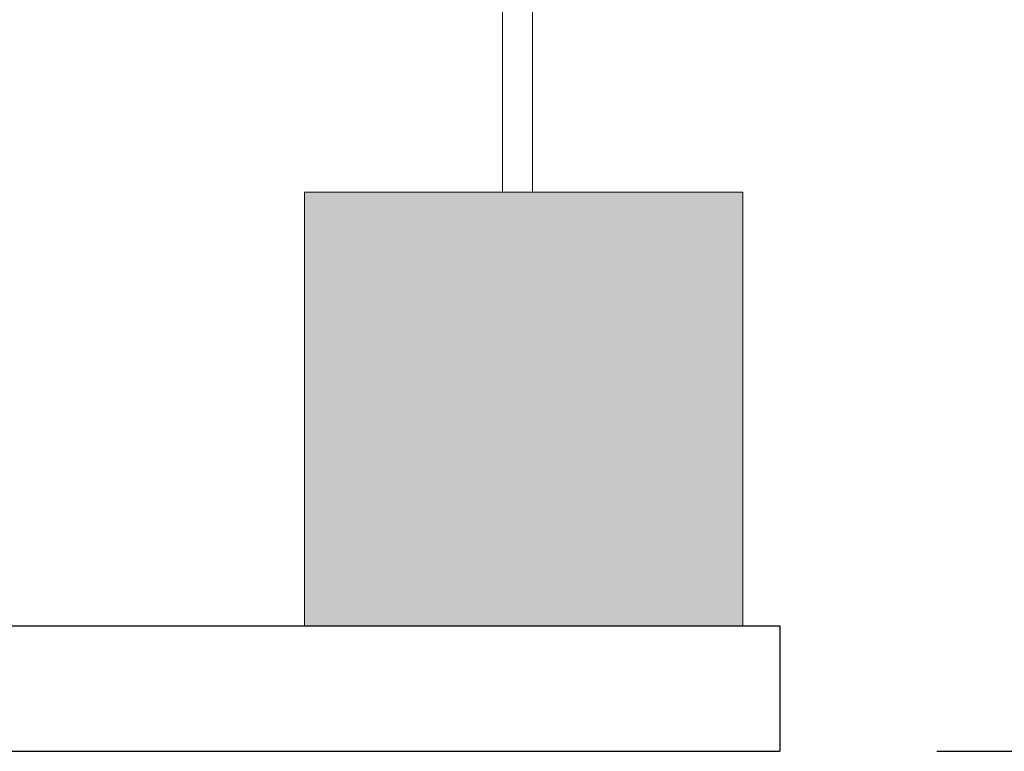
# Model space of a CAD drawing. Units: millimetres. Extents: x 7894 to 8038, y 6851 to 6951.
# Tile 37 of 49: x 7968.188 to 7972.111, y 6922.628 to 6925.542. Entities that reach past the tile are written whole.
import ezdxf

# ---------------------------------------------------------------- set-up
doc = ezdxf.new("R2010")
doc.units = ezdxf.units.MM
for name, color, linetype, lineweight in [('A-ANNO-DIMS', 2, 'Continuous', 18), ('A-FURN-ACCS', 8, 'Continuous', 13), ('A-FURN-SHLF', 7, 'Continuous', 30)]:
    doc.layers.add(name, color=color, linetype=linetype, lineweight=lineweight)
doc.layers.add('A-FURN-ACCS-PATT', color=116, linetype='Continuous', lineweight=9, true_color=0x136734)
doc.styles.get("Standard").update_dxf_attribs({"font": 'arial.ttf'})
doc.dimstyles.new('ISO-25', dxfattribs={"dimtxt": 1, "dimasz": 1, "dimexe": 1.25, "dimexo": 0.625, "dimtad": 1, "dimdec": 0, "dimlunit": 4, "dimtxsty": 'Standard', "dimcen": 2.5, "dimclrt": 1, "dimadec": 0, "dimazin": 0, "dimtfac": 1, "dimtdec": 0, "dimtmove": 0, "dimatfit": 3, "dimfxl": 1, "dimarcsym": 0})

# ---------------------------------------------------------------- blocks, each defined once
blk = doc.blocks.new('DISPLAY-LEAF-FINIAL-Z2_152')
for p, q in [((0.7416, 0, 2.1518), (0.7416, 1.0372, 2.1518)), ((0.8605, 0, 2.1518), (0.8605, 0.9923, 2.1518))]:
    blk.add_line(p, q)
blk = doc.blocks.new('*D23')
at = {"layer": 'A-ANNO-DIMS', "color": 0, "lineweight": -2, "transparency": 16777216}
for p, q in [((7940.0888, 6907.098), (7940.0888, 6947.7928)), ((7971.9356, 6928.989), (7971.9356, 6947.7928)), ((7941.0888, 6946.5428), (7970.9356, 6946.5428))]:
    blk.add_line(p, q, dxfattribs=at)
at = {"layer": 'A-ANNO-DIMS', "color": 0, "transparency": 16777216}
for points in [[(7941.0888, 6946.7095), (7941.0888, 6946.3762), (7940.0888, 6946.5428)], [(7970.9356, 6946.7095), (7970.9356, 6946.3762), (7971.9356, 6946.5428)]]:
    blk.add_solid(points, dxfattribs=at)
at = {"layer": 'Defpoints', "color": 0, "transparency": 16777216}
for p in [(7971.9356, 6946.5428), (7971.9356, 6928.364), (7940.0888, 6906.473)]:
    blk.add_point(p, dxfattribs=at)
at = {"layer": 'A-ANNO-DIMS', "color": 1, "transparency": 16777216, "insert": (7956.0122, 6947.6784), "char_height": 1, "attachment_point": 5}
blk.add_mtext('2\'-8"', dxfattribs=at)
blk = doc.blocks.new('*D28')
at = {"layer": 'A-ANNO-DIMS', "color": 0, "lineweight": -2, "transparency": 16777216}
for p, q in [((7960.8854, 6936.8804), (7975.2272, 6936.8804)), ((7973.9772, 6935.8804), (7973.9772, 6923.6283)), ((7971.8421, 6922.6283), (7975.2272, 6922.6283))]:
    blk.add_line(p, q, dxfattribs=at)
at = {"layer": 'A-ANNO-DIMS', "color": 0, "transparency": 16777216}
for points in [[(7973.8105, 6935.8804), (7974.1439, 6935.8804), (7973.9772, 6936.8804)], [(7973.8105, 6923.6283), (7974.1439, 6923.6283), (7973.9772, 6922.6283)]]:
    blk.add_solid(points, dxfattribs=at)
at = {"layer": 'Defpoints', "color": 0, "transparency": 16777216}
for p in [(7960.2604, 6936.8804), (7971.2171, 6922.6283), (7973.9772, 6922.6283)]:
    blk.add_point(p, dxfattribs=at)
at = {"layer": 'A-ANNO-DIMS', "color": 1, "transparency": 16777216, "insert": (7972.8351, 6929.7543), "char_height": 1, "attachment_point": 5, "rotation": 90}
blk.add_mtext('1\'-2 1/2"', dxfattribs=at)
blk = doc.blocks.new('*D31')
at = {"layer": 'A-ANNO-DIMS', "color": 0, "lineweight": -2, "transparency": 16777216}
for p, q in [((7973.9772, 6921.7198), (7973.9772, 6926.628)), ((7949.8107, 6920.7198), (7975.2272, 6920.7198)), ((7973.9772, 6918.7198), (7973.9772, 6920.7198)), ((7950.9654, 6918.7198), (7975.2272, 6918.7198)), ((7973.9772, 6917.7198), (7973.9772, 6916.7198))]:
    blk.add_line(p, q, dxfattribs=at)
at = {"layer": 'A-ANNO-DIMS', "color": 0, "transparency": 16777216}
for points in [[(7973.8105, 6921.7198), (7974.1439, 6921.7198), (7973.9772, 6920.7198)], [(7973.8105, 6917.7198), (7974.1439, 6917.7198), (7973.9772, 6918.7198)]]:
    blk.add_solid(points, dxfattribs=at)
at = {"layer": 'Defpoints', "color": 0, "transparency": 16777216}
for p in [(7949.1857, 6920.7198), (7973.9772, 6920.7198), (7950.3404, 6918.7198)]:
    blk.add_point(p, dxfattribs=at)
at = {"layer": 'A-ANNO-DIMS', "color": 1, "transparency": 16777216, "insert": (7972.8416, 6924.6739), "char_height": 1, "attachment_point": 5, "rotation": 90}
blk.add_mtext('0\'-2"', dxfattribs=at)

msp = doc.modelspace()

# ---------------------------------------------------------------- hatches: boundary and pattern name
at = {"layer": 'A-FURN-ACCS-PATT'}
h = msp.add_hatch(color=256, dxfattribs=at)
h.dxf.hatch_style = 1
h.paths.add_polyline_path([(7947.5161, 6931.8853), (7946.6774, 6931.8853), (7946.5585, 6931.8853), (7945.7683, 6931.8853), (7945.7683, 6930.1581), (7947.5161, 6930.1581)])
h.paths.add_polyline_path([(7947.4851, 6922.447), (7946.6464, 6922.447), (7946.5276, 6922.447), (7945.7373, 6922.447), (7945.7373, 6920.7198), (7947.4851, 6920.7198)])
h.paths.add_polyline_path([(7968.0212, 6935.881), (7967.1825, 6935.881), (7967.0637, 6935.881), (7966.2734, 6935.881), (7966.2734, 6934.1538), (7968.0212, 6934.1538)])
h.paths.add_polyline_path([(7960.6099, 6924.8555), (7959.7712, 6924.8555), (7959.6523, 6924.8555), (7958.862, 6924.8555), (7958.862, 6923.1283), (7960.6099, 6923.1283)])
h.paths.add_polyline_path([(7964.717, 6924.8555), (7963.8783, 6924.8555), (7963.7594, 6924.8555), (7962.9691, 6924.8555), (7962.9691, 6923.1283), (7964.717, 6923.1283)])
h.paths.add_polyline_path([(7971.0698, 6924.8555), (7970.2311, 6924.8555), (7970.1123, 6924.8555), (7969.322, 6924.8555), (7969.322, 6923.1283), (7971.0698, 6923.1283)])
h.paths.add_polyline_path([(7958.5294, 6908.7006), (7957.6907, 6908.7006), (7957.5718, 6908.7006), (7956.7815, 6908.7006), (7956.7815, 6906.9734), (7958.5294, 6906.9734)])

# ---------------------------------------------------------------- linework, layer by layer
at = {"layer": 'A-FURN-ACCS'}
for p, q in [((7969.322, 6923.1283, 2.1518), (7969.322, 6924.8555, 2.1518)), ((7969.322, 6924.8555, 2.1518), (7970.1123, 6924.8555, 2.1518)), ((7970.2311, 6924.8555, 2.1518), (7970.1123, 6924.8555, 2.1518)), ((7970.2311, 6924.8555, 2.1518), (7971.0698, 6924.8555, 2.1518)), ((7971.0698, 6923.1283, 2.1518), (7971.0698, 6924.8555, 2.1518))]:
    msp.add_line(p, q, dxfattribs=at)
at = {"layer": 'A-FURN-SHLF'}
for p, q in [((7953.9136, 6923.1283, -7), (7971.2171, 6923.1283, -7)), ((7971.2171, 6923.1283, -7), (7971.2171, 6922.6283, -7)), ((7953.9136, 6922.6283, -7), (7971.2171, 6922.6283, -7))]:
    msp.add_line(p, q, dxfattribs=at)

# ---------------------------------------------------------------- block references
at = {"layer": 'A-FURN-ACCS'}
msp.add_blockref('DISPLAY-LEAF-FINIAL-Z2_152', (7969.3706, 6924.8555), dxfattribs=at)

# ---------------------------------------------------------------- dimensions: what is measured, and where the dimension line sits
at = {"layer": 'A-ANNO-DIMS'}
dim = msp.add_linear_dim(base=(7971.9356, 6946.5428), p1=(7940.0888, 6906.473), p2=(7971.9356, 6928.364), dimstyle='ISO-25', override={"dimdec": 1, "dimlfac": 1, "dimrnd": 0, "dimzin": 1, "dimdsep": 46, "dimlunit": 4, "dimfrac": 2}, dxfattribs=at)
dim.commit()
dim.dimension.update_dxf_attribs({"geometry": '*D23', "text_midpoint": (7956.0122, 6947.6784)})
for base, p1, p2, picture, middle in [((7973.9772, 6922.6283), (7960.2604, 6936.8804), (7971.2171, 6922.6283), '*D28', (7972.8351, 6929.7543)), ((7973.9772, 6920.7198), (7950.3404, 6918.7198), (7949.1857, 6920.7198), '*D31', (7972.8416, 6924.6739))]:
    dim = msp.add_linear_dim(base=base, p1=p1, p2=p2, angle=90, dimstyle='ISO-25', override={"dimdec": 1, "dimlfac": 1, "dimrnd": 0, "dimzin": 1, "dimdsep": 46, "dimlunit": 4, "dimfrac": 2}, dxfattribs=at)
    dim.commit()
    dim.dimension.update_dxf_attribs({"geometry": picture, "text_midpoint": middle})

doc.saveas('drawing.dxf')
